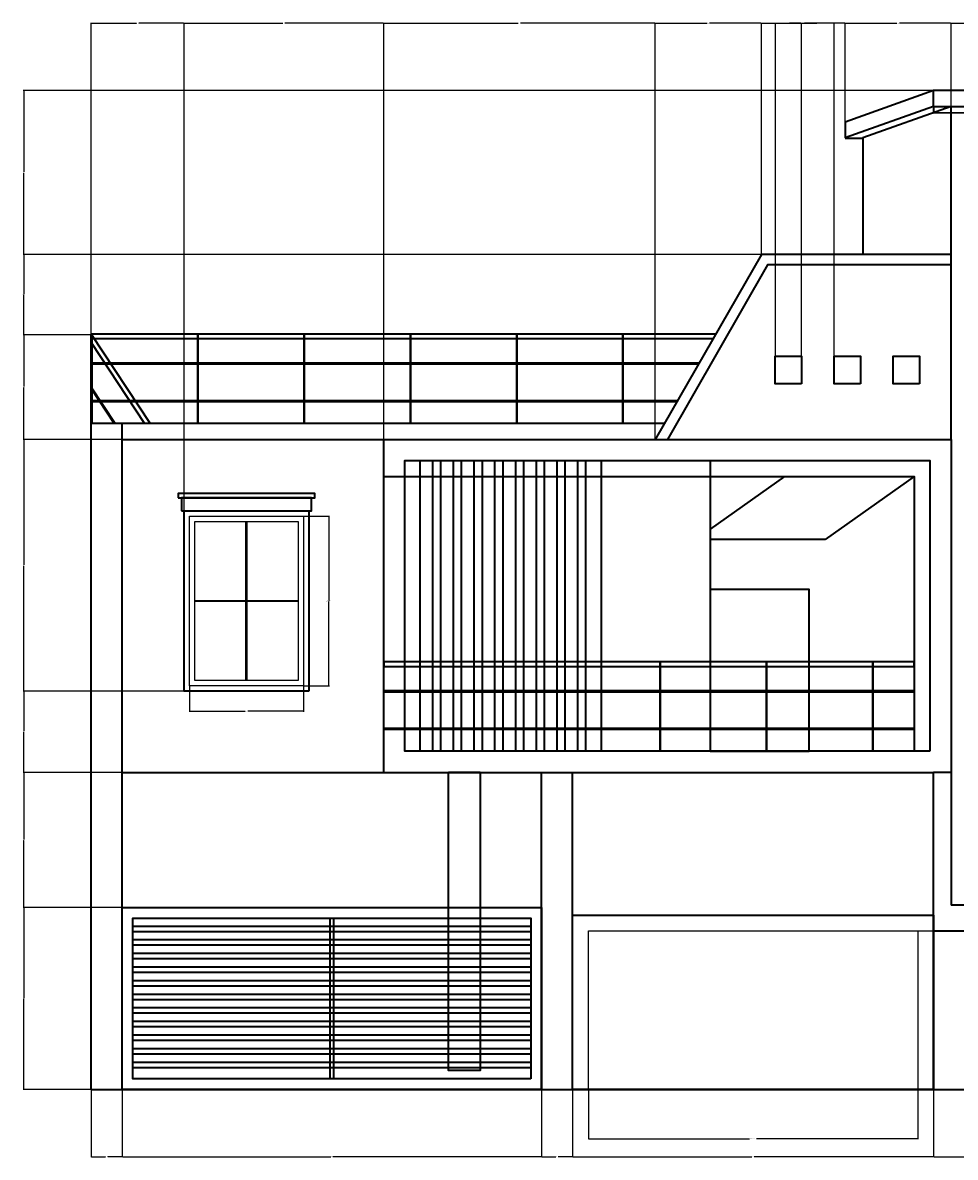
# Model space of a CAD drawing. Units: feet. Extents: x 2415 to 6174, y 866 to 1295.
# Tile 7 of 9: x 3956 to 4309, y 866 to 1295. Entities that reach past the tile are written whole.
import ezdxf

# ---------------------------------------------------------------- set-up
doc = ezdxf.new("R2010")
doc.units = ezdxf.units.FT
for name, color, linetype, lineweight in [('A-ANNO-DIMS', 2, 'Continuous', 18), ('A-DOOR', 4, 'Continuous', 25), ('A-ELEV', 7, 'Continuous', 35), ('A-GLAZ', 4, 'Continuous', 25)]:
    doc.layers.add(name, color=color, linetype=linetype, lineweight=lineweight)
doc.styles.get("Standard").update_dxf_attribs({"font": 'arial.ttf'})
doc.dimstyles.get("Standard").update_dxf_attribs({"dimtxt": 0.18, "dimasz": 0.18, "dimexe": 0.18, "dimexo": 0.0625, "dimgap": 0.09, "dimtad": 0, "dimtih": 1, "dimtoh": 1, "dimdec": 1, "dimzin": 0, "dimdsep": 46, "dimlunit": 3, "dimtxsty": 'Standard', "dimcen": 0.09, "dimadec": 0, "dimazin": 0, "dimtfac": 1, "dimtdec": 1, "dimtofl": 0, "dimtmove": 0, "dimatfit": 3, "dimfxl": 1, "dimtolj": 1, "dimtzin": 0, "dimarcsym": 0})

# ---------------------------------------------------------------- blocks, each defined once
blk = doc.blocks.new('GATE-MAIN')
blk.add_line((0, 60), (124.63, 60))
for points in [[(0, 0), (0, 60)], [(124.63, 60), (124.63, 0)]]:
    blk.add_lwpolyline(points)
blk.add_lwpolyline([(124.63, 0), (0, 0), (0, 60), (124.63, 60)], close=True)
blk = doc.blocks.new('WIN-SMALL')
for points in [[(3333.49, 1044.32), (3290.35, 1044.32), (3290.35, 1108.53), (3333.49, 1108.53)], [(3331.49, 1046.32), (3292.35, 1046.32), (3292.35, 1106.53), (3331.49, 1106.53)], [(3311.72, 1106.53), (3312.12, 1106.53), (3312.12, 1046.32), (3311.72, 1046.32)]]:
    blk.add_lwpolyline(points, close=True)
for points in [[(3292.35, 1076.62), (3331.49, 1076.62)], [(3331.49, 1076.22), (3292.35, 1076.22)]]:
    blk.add_lwpolyline(points)
blk = doc.blocks.new('*D15')
at = {"layer": 'A-ANNO-DIMS', "color": 0, "lineweight": -2, "transparency": 16777216}
for p, q in [((4170.36, 891.54), (4170.36, 872.73)), ((4294.99, 891.54), (4294.99, 872.73)), ((4170.54, 872.91), (4231.36, 872.91)), ((4294.81, 872.91), (4234, 872.91))]:
    blk.add_line(p, q, dxfattribs=at)
at = {"layer": 'A-ANNO-DIMS', "color": 0, "transparency": 16777216}
for points in [[(4170.54, 872.94), (4170.54, 872.88), (4170.36, 872.91)], [(4294.81, 872.94), (4294.81, 872.88), (4294.99, 872.91)]]:
    blk.add_solid(points, dxfattribs=at)
at = {"layer": 'Defpoints', "color": 0, "transparency": 16777216}
for p in [(4170.36, 891.6), (4294.99, 891.6), (4294.99, 872.91)]:
    blk.add_point(p, dxfattribs=at)
at = {"layer": 'A-ANNO-DIMS', "color": 0, "transparency": 16777216, "insert": (4232.68, 872.91), "char_height": 0.18, "attachment_point": 5}
blk.add_mtext('\\A1;MAIN GATE 125 TYP.', dxfattribs=at)
blk = doc.blocks.new('*D16')
at = {"layer": 'A-ANNO-DIMS', "color": 0, "lineweight": -2, "transparency": 16777216}
for p, q in [((4295.05, 951.6), (4313.86, 951.6)), ((4313.68, 951.42), (4313.68, 921.78)), ((4313.68, 891.78), (4313.68, 921.42)), ((4295.05, 891.6), (4313.86, 891.6))]:
    blk.add_line(p, q, dxfattribs=at)
at = {"layer": 'A-ANNO-DIMS', "color": 0, "transparency": 16777216}
for points in [[(4313.65, 951.42), (4313.71, 951.42), (4313.68, 951.6)], [(4313.65, 891.78), (4313.71, 891.78), (4313.68, 891.6)]]:
    blk.add_solid(points, dxfattribs=at)
at = {"layer": 'Defpoints', "color": 0, "transparency": 16777216}
for p in [(4294.99, 951.6), (4313.68, 951.6), (4294.99, 891.6)]:
    blk.add_point(p, dxfattribs=at)
at = {"layer": 'A-ANNO-DIMS', "color": 0, "transparency": 16777216, "insert": (4313.68, 921.6), "char_height": 0.18, "attachment_point": 5}
blk.add_mtext('\\A1;60 TYP.', dxfattribs=at)
blk = doc.blocks.new('*D17')
at = {"layer": 'A-ANNO-DIMS', "color": 0, "lineweight": -2, "transparency": 16777216}
for p, q in [((4062.61, 1108.53), (4072.36, 1108.53)), ((4072.18, 1108.35), (4072.18, 1076.61)), ((4072.18, 1044.5), (4072.18, 1076.24)), ((4062.61, 1044.32), (4072.36, 1044.32))]:
    blk.add_line(p, q, dxfattribs=at)
at = {"layer": 'A-ANNO-DIMS', "color": 0, "transparency": 16777216}
for points in [[(4072.15, 1108.35), (4072.21, 1108.35), (4072.18, 1108.53)], [(4072.15, 1044.5), (4072.21, 1044.5), (4072.18, 1044.32)]]:
    blk.add_solid(points, dxfattribs=at)
at = {"layer": 'Defpoints', "color": 0, "transparency": 16777216}
for p in [(4062.54, 1108.53), (4072.18, 1108.53), (4062.54, 1044.32)]:
    blk.add_point(p, dxfattribs=at)
at = {"layer": 'A-ANNO-DIMS', "color": 0, "transparency": 16777216, "insert": (4072.18, 1076.42), "char_height": 0.18, "attachment_point": 5}
blk.add_mtext('\\A1;WINDOW 64 TYP.', dxfattribs=at)
blk = doc.blocks.new('*D18')
at = {"layer": 'A-ANNO-DIMS', "color": 0, "lineweight": -2, "transparency": 16777216}
for p, q in [((4019.4, 1044.26), (4019.4, 1034.51)), ((4062.54, 1044.26), (4062.54, 1034.51)), ((4019.58, 1034.69), (4040.44, 1034.69)), ((4062.36, 1034.69), (4041.5, 1034.69))]:
    blk.add_line(p, q, dxfattribs=at)
at = {"layer": 'A-ANNO-DIMS', "color": 0, "transparency": 16777216}
for points in [[(4019.58, 1034.72), (4019.58, 1034.66), (4019.4, 1034.69)], [(4062.36, 1034.72), (4062.36, 1034.66), (4062.54, 1034.69)]]:
    blk.add_solid(points, dxfattribs=at)
at = {"layer": 'Defpoints', "color": 0, "transparency": 16777216}
for p in [(4019.4, 1044.32), (4062.54, 1044.32), (4062.54, 1034.69)]:
    blk.add_point(p, dxfattribs=at)
at = {"layer": 'A-ANNO-DIMS', "color": 0, "transparency": 16777216, "insert": (4040.97, 1034.69), "char_height": 0.18, "attachment_point": 5}
blk.add_mtext('\\A1;43 TYP.', dxfattribs=at)
blk = doc.blocks.new('*D19')
at = {"layer": 'A-ANNO-DIMS', "color": 0, "lineweight": -2, "transparency": 16777216}
for p, q in [((3982.18, 891.54), (3982.18, 865.92)), ((3993.97, 891.54), (3993.97, 865.92)), ((3982.36, 866.1), (3987.62, 866.1)), ((3993.79, 866.1), (3988.53, 866.1))]:
    blk.add_line(p, q, dxfattribs=at)
at = {"layer": 'A-ANNO-DIMS', "color": 0, "transparency": 16777216}
for points in [[(3982.36, 866.13), (3982.36, 866.07), (3982.18, 866.1)], [(3993.79, 866.13), (3993.79, 866.07), (3993.97, 866.1)]]:
    blk.add_solid(points, dxfattribs=at)
at = {"layer": 'Defpoints', "color": 0, "transparency": 16777216}
for p in [(3982.18, 891.6), (3993.97, 891.6), (3993.97, 866.1)]:
    blk.add_point(p, dxfattribs=at)
at = {"layer": 'A-ANNO-DIMS', "color": 0, "transparency": 16777216, "insert": (3988.08, 866.1), "char_height": 0.18, "attachment_point": 5}
blk.add_mtext('\\A1;11.787', dxfattribs=at)
blk = doc.blocks.new('*D20')
at = {"layer": 'A-ANNO-DIMS', "color": 0, "lineweight": -2, "transparency": 16777216}
for p, q in [((3993.97, 891.54), (3993.97, 865.92)), ((4152.58, 891.54), (4152.58, 865.92)), ((3994.15, 866.1), (4072.89, 866.1)), ((4152.4, 866.1), (4073.66, 866.1))]:
    blk.add_line(p, q, dxfattribs=at)
at = {"layer": 'A-ANNO-DIMS', "color": 0, "transparency": 16777216}
for points in [[(3994.15, 866.13), (3994.15, 866.07), (3993.97, 866.1)], [(4152.4, 866.13), (4152.4, 866.07), (4152.58, 866.1)]]:
    blk.add_solid(points, dxfattribs=at)
at = {"layer": 'Defpoints', "color": 0, "transparency": 16777216}
for p in [(3993.97, 891.6), (4152.58, 891.6), (4152.58, 866.1)]:
    blk.add_point(p, dxfattribs=at)
at = {"layer": 'A-ANNO-DIMS', "color": 0, "transparency": 16777216, "insert": (4073.27, 866.1), "char_height": 0.18, "attachment_point": 5}
blk.add_mtext('\\A1;158.6', dxfattribs=at)
blk = doc.blocks.new('*D21')
at = {"layer": 'A-ANNO-DIMS', "color": 0, "lineweight": -2, "transparency": 16777216}
for p, q in [((4152.58, 891.54), (4152.58, 865.92)), ((4164.36, 891.54), (4164.36, 865.92)), ((4152.76, 866.1), (4158.01, 866.1)), ((4164.18, 866.1), (4158.93, 866.1))]:
    blk.add_line(p, q, dxfattribs=at)
at = {"layer": 'A-ANNO-DIMS', "color": 0, "transparency": 16777216}
for points in [[(4152.76, 866.13), (4152.76, 866.07), (4152.58, 866.1)], [(4164.18, 866.13), (4164.18, 866.07), (4164.36, 866.1)]]:
    blk.add_solid(points, dxfattribs=at)
at = {"layer": 'Defpoints', "color": 0, "transparency": 16777216}
for p in [(4152.58, 891.6), (4164.36, 891.6), (4164.36, 866.1)]:
    blk.add_point(p, dxfattribs=at)
at = {"layer": 'A-ANNO-DIMS', "color": 0, "transparency": 16777216, "insert": (4158.47, 866.1), "char_height": 0.18, "attachment_point": 5}
blk.add_mtext('\\A1;11.787', dxfattribs=at)
blk = doc.blocks.new('*D22')
at = {"layer": 'A-ANNO-DIMS', "color": 0, "lineweight": -2, "transparency": 16777216}
for p, q in [((4164.36, 891.54), (4164.36, 865.92)), ((4300.99, 891.54), (4300.99, 865.92)), ((4164.54, 866.1), (4232.22, 866.1)), ((4300.81, 866.1), (4233.13, 866.1))]:
    blk.add_line(p, q, dxfattribs=at)
at = {"layer": 'A-ANNO-DIMS', "color": 0, "transparency": 16777216}
for points in [[(4164.54, 866.13), (4164.54, 866.07), (4164.36, 866.1)], [(4300.81, 866.13), (4300.81, 866.07), (4300.99, 866.1)]]:
    blk.add_solid(points, dxfattribs=at)
at = {"layer": 'Defpoints', "color": 0, "transparency": 16777216}
for p in [(4164.36, 891.6), (4300.99, 891.6), (4300.99, 866.1)]:
    blk.add_point(p, dxfattribs=at)
at = {"layer": 'A-ANNO-DIMS', "color": 0, "transparency": 16777216, "insert": (4232.68, 866.1), "char_height": 0.18, "attachment_point": 5}
blk.add_mtext('\\A1;136.63', dxfattribs=at)
blk = doc.blocks.new('*D23')
at = {"layer": 'A-ANNO-DIMS', "color": 0, "lineweight": -2, "transparency": 16777216}
for p, q in [((4300.99, 891.54), (4300.99, 865.92)), ((4330.05, 891.54), (4330.05, 865.92)), ((4301.17, 866.1), (4315.13, 866.1)), ((4329.87, 866.1), (4315.92, 866.1))]:
    blk.add_line(p, q, dxfattribs=at)
at = {"layer": 'A-ANNO-DIMS', "color": 0, "transparency": 16777216}
for points in [[(4301.17, 866.13), (4301.17, 866.07), (4300.99, 866.1)], [(4329.87, 866.13), (4329.87, 866.07), (4330.05, 866.1)]]:
    blk.add_solid(points, dxfattribs=at)
at = {"layer": 'Defpoints', "color": 0, "transparency": 16777216}
for p in [(4300.99, 891.6), (4330.05, 891.6), (4330.05, 866.1)]:
    blk.add_point(p, dxfattribs=at)
at = {"layer": 'A-ANNO-DIMS', "color": 0, "transparency": 16777216, "insert": (4315.52, 866.1), "char_height": 0.18, "attachment_point": 5}
blk.add_mtext('\\A1;29.06', dxfattribs=at)
blk = doc.blocks.new('*D27')
at = {"layer": 'A-ANNO-DIMS', "color": 0, "lineweight": -2, "transparency": 16777216}
for p, q in [((3982.18, 1177.2), (3982.18, 1295.28)), ((3982.36, 1295.1), (3999.33, 1295.1)), ((4017.22, 1295.1), (4000.26, 1295.1)), ((4017.4, 1042.38), (4017.4, 1295.28))]:
    blk.add_line(p, q, dxfattribs=at)
at = {"layer": 'A-ANNO-DIMS', "color": 0, "transparency": 16777216}
for points in [[(3982.36, 1295.13), (3982.36, 1295.07), (3982.18, 1295.1)], [(4017.22, 1295.13), (4017.22, 1295.07), (4017.4, 1295.1)]]:
    blk.add_solid(points, dxfattribs=at)
at = {"layer": 'Defpoints', "color": 0, "transparency": 16777216}
for p in [(4017.4, 1295.1), (3982.18, 1177.14), (4017.4, 1042.32)]:
    blk.add_point(p, dxfattribs=at)
at = {"layer": 'A-ANNO-DIMS', "color": 0, "transparency": 16777216, "insert": (3999.79, 1295.1), "char_height": 0.18, "attachment_point": 5}
blk.add_mtext('\\A1;35.216', dxfattribs=at)
blk = doc.blocks.new('*D28')
at = {"layer": 'A-ANNO-DIMS', "color": 0, "lineweight": -2, "transparency": 16777216}
for p, q in [((4017.4, 1042.38), (4017.4, 1295.28)), ((4017.58, 1295.1), (4054.77, 1295.1)), ((4092.74, 1295.1), (4055.55, 1295.1)), ((4092.92, 1137.66), (4092.92, 1295.28))]:
    blk.add_line(p, q, dxfattribs=at)
at = {"layer": 'A-ANNO-DIMS', "color": 0, "transparency": 16777216}
for points in [[(4017.58, 1295.13), (4017.58, 1295.07), (4017.4, 1295.1)], [(4092.74, 1295.13), (4092.74, 1295.07), (4092.92, 1295.1)]]:
    blk.add_solid(points, dxfattribs=at)
at = {"layer": 'Defpoints', "color": 0, "transparency": 16777216}
for p in [(4092.92, 1295.1), (4092.92, 1137.6), (4017.4, 1042.32)]:
    blk.add_point(p, dxfattribs=at)
at = {"layer": 'A-ANNO-DIMS', "color": 0, "transparency": 16777216, "insert": (4055.16, 1295.1), "char_height": 0.18, "attachment_point": 5}
blk.add_mtext('\\A1;75.52', dxfattribs=at)
blk = doc.blocks.new('*D29')
at = {"layer": 'A-ANNO-DIMS', "color": 0, "lineweight": -2, "transparency": 16777216}
for p, q in [((4092.92, 1137.66), (4092.92, 1295.28)), ((4093.1, 1295.1), (4143.83, 1295.1)), ((4195.48, 1295.1), (4144.74, 1295.1)), ((4195.66, 1137.66), (4195.66, 1295.28))]:
    blk.add_line(p, q, dxfattribs=at)
at = {"layer": 'A-ANNO-DIMS', "color": 0, "transparency": 16777216}
for points in [[(4093.1, 1295.13), (4093.1, 1295.07), (4092.92, 1295.1)], [(4195.48, 1295.13), (4195.48, 1295.07), (4195.66, 1295.1)]]:
    blk.add_solid(points, dxfattribs=at)
at = {"layer": 'Defpoints', "color": 0, "transparency": 16777216}
for p in [(4195.66, 1295.1), (4092.92, 1137.6), (4195.66, 1137.6)]:
    blk.add_point(p, dxfattribs=at)
at = {"layer": 'A-ANNO-DIMS', "color": 0, "transparency": 16777216, "insert": (4144.29, 1295.1), "char_height": 0.18, "attachment_point": 5}
blk.add_mtext('\\A1;102.73', dxfattribs=at)
blk = doc.blocks.new('*D30')
at = {"layer": 'A-ANNO-DIMS', "color": 0, "lineweight": -2, "transparency": 16777216}
for p, q in [((4195.66, 1137.66), (4195.66, 1295.28)), ((4195.84, 1295.1), (4215.35, 1295.1)), ((4235.67, 1295.1), (4216.15, 1295.1)), ((4235.85, 1207.66), (4235.85, 1295.28))]:
    blk.add_line(p, q, dxfattribs=at)
at = {"layer": 'A-ANNO-DIMS', "color": 0, "transparency": 16777216}
for points in [[(4195.84, 1295.13), (4195.84, 1295.07), (4195.66, 1295.1)], [(4235.67, 1295.13), (4235.67, 1295.07), (4235.85, 1295.1)]]:
    blk.add_solid(points, dxfattribs=at)
at = {"layer": 'Defpoints', "color": 0, "transparency": 16777216}
for p in [(4235.85, 1295.1), (4235.85, 1207.6), (4195.66, 1137.6)]:
    blk.add_point(p, dxfattribs=at)
at = {"layer": 'A-ANNO-DIMS', "color": 0, "transparency": 16777216, "insert": (4215.75, 1295.1), "char_height": 0.18, "attachment_point": 5}
blk.add_mtext('\\A1;40.19', dxfattribs=at)
blk = doc.blocks.new('*D31')
at = {"layer": 'A-ANNO-DIMS', "color": 0, "lineweight": -2, "transparency": 16777216}
for p, q in [((4235.85, 1207.66), (4235.85, 1295.28)), ((4236.03, 1295.1), (4251.31, 1295.1)), ((4267.39, 1295.1), (4252.1, 1295.1)), ((4267.57, 1257.71), (4267.57, 1295.28))]:
    blk.add_line(p, q, dxfattribs=at)
at = {"layer": 'A-ANNO-DIMS', "color": 0, "transparency": 16777216}
for points in [[(4236.03, 1295.13), (4236.03, 1295.07), (4235.85, 1295.1)], [(4267.39, 1295.13), (4267.39, 1295.07), (4267.57, 1295.1)]]:
    blk.add_solid(points, dxfattribs=at)
at = {"layer": 'Defpoints', "color": 0, "transparency": 16777216}
for p in [(4267.57, 1295.1), (4267.57, 1257.64), (4235.85, 1207.6)]:
    blk.add_point(p, dxfattribs=at)
at = {"layer": 'A-ANNO-DIMS', "color": 0, "transparency": 16777216, "insert": (4251.71, 1295.1), "char_height": 0.18, "attachment_point": 5}
blk.add_mtext('\\A1;31.72', dxfattribs=at)
blk = doc.blocks.new('*D32')
at = {"layer": 'A-ANNO-DIMS', "color": 0, "lineweight": -2, "transparency": 16777216}
for p, q in [((4267.57, 1257.71), (4267.57, 1295.28)), ((4267.75, 1295.1), (4287.12, 1295.1)), ((4307.43, 1295.1), (4288.06, 1295.1)), ((4307.61, 1263.66), (4307.61, 1295.28))]:
    blk.add_line(p, q, dxfattribs=at)
at = {"layer": 'A-ANNO-DIMS', "color": 0, "transparency": 16777216}
for points in [[(4267.75, 1295.13), (4267.75, 1295.07), (4267.57, 1295.1)], [(4307.43, 1295.13), (4307.43, 1295.07), (4307.61, 1295.1)]]:
    blk.add_solid(points, dxfattribs=at)
at = {"layer": 'Defpoints', "color": 0, "transparency": 16777216}
for p in [(4307.61, 1295.1), (4307.61, 1263.6), (4267.57, 1257.64)]:
    blk.add_point(p, dxfattribs=at)
at = {"layer": 'A-ANNO-DIMS', "color": 0, "transparency": 16777216, "insert": (4287.59, 1295.1), "char_height": 0.18, "attachment_point": 5}
blk.add_mtext('\\A1;40.046', dxfattribs=at)
blk = doc.blocks.new('*D33')
at = {"layer": 'A-ANNO-DIMS', "color": 0, "lineweight": -2, "transparency": 16777216}
for p, q in [((4307.61, 1263.66), (4307.61, 1295.28)), ((4307.79, 1295.1), (4318.98, 1295.1)), ((4331.09, 1295.1), (4319.91, 1295.1)), ((4331.27, 1239.13), (4331.27, 1295.28))]:
    blk.add_line(p, q, dxfattribs=at)
at = {"layer": 'A-ANNO-DIMS', "color": 0, "transparency": 16777216}
for points in [[(4307.79, 1295.13), (4307.79, 1295.07), (4307.61, 1295.1)], [(4331.09, 1295.13), (4331.09, 1295.07), (4331.27, 1295.1)]]:
    blk.add_solid(points, dxfattribs=at)
at = {"layer": 'Defpoints', "color": 0, "transparency": 16777216}
for p in [(4331.27, 1295.1), (4307.61, 1263.6), (4331.27, 1239.07)]:
    blk.add_point(p, dxfattribs=at)
at = {"layer": 'A-ANNO-DIMS', "color": 0, "transparency": 16777216, "insert": (4319.44, 1295.1), "char_height": 0.18, "attachment_point": 5}
blk.add_mtext('\\A1;23.657', dxfattribs=at)
blk = doc.blocks.new('*D38')
at = {"layer": 'A-ANNO-DIMS', "color": 0, "lineweight": -2, "transparency": 16777216}
for p, q in [((3993.91, 960.43), (3956.5, 960.43)), ((3956.68, 960.25), (3956.68, 926.2)), ((3956.68, 891.78), (3956.68, 925.83)), ((3993.91, 891.6), (3956.5, 891.6))]:
    blk.add_line(p, q, dxfattribs=at)
at = {"layer": 'A-ANNO-DIMS', "color": 0, "transparency": 16777216}
for points in [[(3956.65, 960.25), (3956.71, 960.25), (3956.68, 960.43)], [(3956.65, 891.78), (3956.71, 891.78), (3956.68, 891.6)]]:
    blk.add_solid(points, dxfattribs=at)
at = {"layer": 'Defpoints', "color": 0, "transparency": 16777216}
for p in [(3956.68, 960.43), (3993.97, 960.43), (3993.97, 891.6)]:
    blk.add_point(p, dxfattribs=at)
at = {"layer": 'A-ANNO-DIMS', "color": 0, "transparency": 16777216, "insert": (3956.68, 926.02), "char_height": 0.18, "attachment_point": 5}
blk.add_mtext('\\A1;68.83', dxfattribs=at)
blk = doc.blocks.new('*D39')
at = {"layer": 'A-ANNO-DIMS', "color": 0, "lineweight": -2, "transparency": 16777216}
for p, q in [((3993.91, 1011.6), (3956.5, 1011.6)), ((3956.68, 1011.42), (3956.68, 986.2)), ((3956.68, 960.61), (3956.68, 985.83)), ((3993.91, 960.43), (3956.5, 960.43))]:
    blk.add_line(p, q, dxfattribs=at)
at = {"layer": 'A-ANNO-DIMS', "color": 0, "transparency": 16777216}
for points in [[(3956.65, 1011.42), (3956.71, 1011.42), (3956.68, 1011.6)], [(3956.65, 960.61), (3956.71, 960.61), (3956.68, 960.43)]]:
    blk.add_solid(points, dxfattribs=at)
at = {"layer": 'Defpoints', "color": 0, "transparency": 16777216}
for p in [(3956.68, 1011.6), (3993.97, 1011.6), (3993.97, 960.43)]:
    blk.add_point(p, dxfattribs=at)
at = {"layer": 'A-ANNO-DIMS', "color": 0, "transparency": 16777216, "insert": (3956.68, 986.02), "char_height": 0.18, "attachment_point": 5}
blk.add_mtext('\\A1;51.17', dxfattribs=at)
blk = doc.blocks.new('*D40')
at = {"layer": 'A-ANNO-DIMS', "color": 0, "lineweight": -2, "transparency": 16777216}
for p, q in [((4017.34, 1042.32), (3956.5, 1042.32)), ((3956.68, 1042.14), (3956.68, 1027.14)), ((3956.68, 1011.78), (3956.68, 1026.78)), ((3993.91, 1011.6), (3956.5, 1011.6))]:
    blk.add_line(p, q, dxfattribs=at)
at = {"layer": 'A-ANNO-DIMS', "color": 0, "transparency": 16777216}
for points in [[(3956.65, 1042.14), (3956.71, 1042.14), (3956.68, 1042.32)], [(3956.65, 1011.78), (3956.71, 1011.78), (3956.68, 1011.6)]]:
    blk.add_solid(points, dxfattribs=at)
at = {"layer": 'Defpoints', "color": 0, "transparency": 16777216}
for p in [(3956.68, 1042.32), (4017.4, 1042.32), (3993.97, 1011.6)]:
    blk.add_point(p, dxfattribs=at)
at = {"layer": 'A-ANNO-DIMS', "color": 0, "transparency": 16777216, "insert": (3956.68, 1026.96), "char_height": 0.18, "attachment_point": 5}
blk.add_mtext('\\A1;30.72', dxfattribs=at)
blk = doc.blocks.new('*D41')
at = {"layer": 'A-ANNO-DIMS', "color": 0, "lineweight": -2, "transparency": 16777216}
for p, q in [((4092.86, 1137.6), (3956.5, 1137.6)), ((3956.68, 1137.42), (3956.68, 1090.14)), ((3956.68, 1042.5), (3956.68, 1089.78)), ((4017.34, 1042.32), (3956.5, 1042.32))]:
    blk.add_line(p, q, dxfattribs=at)
at = {"layer": 'A-ANNO-DIMS', "color": 0, "transparency": 16777216}
for points in [[(3956.65, 1137.42), (3956.71, 1137.42), (3956.68, 1137.6)], [(3956.65, 1042.5), (3956.71, 1042.5), (3956.68, 1042.32)]]:
    blk.add_solid(points, dxfattribs=at)
at = {"layer": 'Defpoints', "color": 0, "transparency": 16777216}
for p in [(3956.68, 1137.6), (4092.92, 1137.6), (4017.4, 1042.32)]:
    blk.add_point(p, dxfattribs=at)
at = {"layer": 'A-ANNO-DIMS', "color": 0, "transparency": 16777216, "insert": (3956.68, 1089.96), "char_height": 0.18, "attachment_point": 5}
blk.add_mtext('\\A1;95.28', dxfattribs=at)
blk = doc.blocks.new('*D42')
at = {"layer": 'A-ANNO-DIMS', "color": 0, "lineweight": -2, "transparency": 16777216}
for p, q in [((3982.12, 1177.14), (3956.5, 1177.14)), ((3956.68, 1176.96), (3956.68, 1157.55)), ((3956.68, 1137.78), (3956.68, 1157.19)), ((4092.86, 1137.6), (3956.5, 1137.6))]:
    blk.add_line(p, q, dxfattribs=at)
at = {"layer": 'A-ANNO-DIMS', "color": 0, "transparency": 16777216}
for points in [[(3956.65, 1176.96), (3956.71, 1176.96), (3956.68, 1177.14)], [(3956.65, 1137.78), (3956.71, 1137.78), (3956.68, 1137.6)]]:
    blk.add_solid(points, dxfattribs=at)
at = {"layer": 'Defpoints', "color": 0, "transparency": 16777216}
for p in [(3956.68, 1177.14), (3982.18, 1177.14), (4092.92, 1137.6)]:
    blk.add_point(p, dxfattribs=at)
at = {"layer": 'A-ANNO-DIMS', "color": 0, "transparency": 16777216, "insert": (3956.68, 1157.37), "char_height": 0.18, "attachment_point": 5}
blk.add_mtext('\\A1;39.54', dxfattribs=at)
blk = doc.blocks.new('*D43')
at = {"layer": 'A-ANNO-DIMS', "color": 0, "lineweight": -2, "transparency": 16777216}
for p, q in [((4235.78, 1207.6), (3956.5, 1207.6)), ((3956.68, 1207.42), (3956.68, 1192.55)), ((3956.68, 1177.32), (3956.68, 1192.19)), ((3982.12, 1177.14), (3956.5, 1177.14))]:
    blk.add_line(p, q, dxfattribs=at)
at = {"layer": 'A-ANNO-DIMS', "color": 0, "transparency": 16777216}
for points in [[(3956.65, 1207.42), (3956.71, 1207.42), (3956.68, 1207.6)], [(3956.65, 1177.32), (3956.71, 1177.32), (3956.68, 1177.14)]]:
    blk.add_solid(points, dxfattribs=at)
at = {"layer": 'Defpoints', "color": 0, "transparency": 16777216}
for p in [(3956.68, 1207.6), (4235.85, 1207.6), (3982.18, 1177.14)]:
    blk.add_point(p, dxfattribs=at)
at = {"layer": 'A-ANNO-DIMS', "color": 0, "transparency": 16777216, "insert": (3956.68, 1192.37), "char_height": 0.18, "attachment_point": 5}
blk.add_mtext('\\A1;30.457', dxfattribs=at)
blk = doc.blocks.new('*D44')
at = {"layer": 'A-ANNO-DIMS', "color": 0, "lineweight": -2, "transparency": 16777216}
for p, q in [((4300.93, 1269.6), (3956.5, 1269.6)), ((3956.68, 1269.42), (3956.68, 1238.78)), ((3956.68, 1207.78), (3956.68, 1238.42)), ((4235.78, 1207.6), (3956.5, 1207.6))]:
    blk.add_line(p, q, dxfattribs=at)
at = {"layer": 'A-ANNO-DIMS', "color": 0, "transparency": 16777216}
for points in [[(3956.65, 1269.42), (3956.71, 1269.42), (3956.68, 1269.6)], [(3956.65, 1207.78), (3956.71, 1207.78), (3956.68, 1207.6)]]:
    blk.add_solid(points, dxfattribs=at)
at = {"layer": 'Defpoints', "color": 0, "transparency": 16777216}
for p in [(3956.68, 1269.6), (4300.99, 1269.6), (4235.85, 1207.6)]:
    blk.add_point(p, dxfattribs=at)
at = {"layer": 'A-ANNO-DIMS', "color": 0, "transparency": 16777216, "insert": (3956.68, 1238.6), "char_height": 0.18, "attachment_point": 5}
blk.add_mtext('\\A1;62', dxfattribs=at)
blk = doc.blocks.new('*D51')
at = {"layer": 'A-ANNO-DIMS', "color": 0, "lineweight": -2, "transparency": 16777216}
for p, q in [((4241.11, 1169.09), (4241.11, 1295.28)), ((4241.29, 1295.1), (4245.66, 1295.1)), ((4250.81, 1295.1), (4246.44, 1295.1)), ((4250.99, 1169.09), (4250.99, 1295.28))]:
    blk.add_line(p, q, dxfattribs=at)
at = {"layer": 'A-ANNO-DIMS', "color": 0, "transparency": 16777216}
for points in [[(4241.29, 1295.13), (4241.29, 1295.07), (4241.11, 1295.1)], [(4250.81, 1295.13), (4250.81, 1295.07), (4250.99, 1295.1)]]:
    blk.add_solid(points, dxfattribs=at)
at = {"layer": 'Defpoints', "color": 0, "transparency": 16777216}
for p in [(4250.99, 1295.1), (4241.11, 1169.03), (4250.99, 1169.03)]:
    blk.add_point(p, dxfattribs=at)
at = {"layer": 'A-ANNO-DIMS', "color": 0, "transparency": 16777216, "insert": (4246.05, 1295.1), "char_height": 0.18, "attachment_point": 5}
blk.add_mtext('\\A1;9.886', dxfattribs=at)
blk = doc.blocks.new('*D52')
at = {"layer": 'A-ANNO-DIMS', "color": 0, "lineweight": -2, "transparency": 16777216}
for p, q in [((4250.99, 1158.74), (4250.99, 1295.28)), ((4251.17, 1295.1), (4256.76, 1295.1)), ((4263.25, 1295.1), (4257.67, 1295.1)), ((4263.43, 1158.74), (4263.43, 1295.28))]:
    blk.add_line(p, q, dxfattribs=at)
at = {"layer": 'A-ANNO-DIMS', "color": 0, "transparency": 16777216}
for points in [[(4251.17, 1295.13), (4251.17, 1295.07), (4250.99, 1295.1)], [(4263.25, 1295.13), (4263.25, 1295.07), (4263.43, 1295.1)]]:
    blk.add_solid(points, dxfattribs=at)
at = {"layer": 'Defpoints', "color": 0, "transparency": 16777216}
for p in [(4263.43, 1295.1), (4250.99, 1158.67), (4263.43, 1158.67)]:
    blk.add_point(p, dxfattribs=at)
at = {"layer": 'A-ANNO-DIMS', "color": 0, "transparency": 16777216, "insert": (4257.21, 1295.1), "char_height": 0.18, "attachment_point": 5}
blk.add_mtext('\\A1;12.438', dxfattribs=at)

msp = doc.modelspace()

# ---------------------------------------------------------------- linework, layer by layer
at = {"layer": 'A-ELEV'}
for p, q in [((4300.9903, 1269.5992), (4267.5678, 1257.6449)), ((4419.1468, 1269.5992), (4300.9903, 1269.5992)), ((4300.9903, 1263.5992), (4300.9903, 1269.5992)), ((4300.9903, 1263.5992), (4267.5678, 1251.6449)), ((4307.6134, 1263.5992), (4274.1909, 1251.6449)), ((4300.9903, 1263.5992), (4419.1468, 1263.5992)), ((4300.9903, 1263.5992), (4300.9903, 1261.2303)), ((4307.6134, 1137.5992), (4307.6134, 1263.5992)), ((4300.9903, 1261.2303), (4411.1278, 1261.2628)), ((4267.5678, 1257.6449), (4267.5678, 1251.6449)), ((4267.5678, 1251.6449), (4267.6022, 1251.5295)), ((4267.5678, 1251.5295), (4274.1909, 1251.5295)), ((4273.8049, 1251.5295), (4274.1909, 1251.6449)), ((4274.1909, 1251.6449), (4274.1909, 1207.5992)), ((3982.1845, 1143.5993), (3982.1845, 1177.4585)), ((3982.1845, 1177.4585), (4004.5183, 1143.5993)), ((3982.1845, 891.5992), (3982.1845, 1143.5993)), ((3993.9716, 1143.5993), (3982.1845, 1143.5993)), ((4199.1004, 1143.5993), (3993.9716, 1143.5993)), ((3993.9716, 1137.5992), (4307.6134, 1137.5992)), ((4092.9223, 1011.5992), (4092.9223, 1137.5992)), ((4307.6134, 1137.5992), (4307.6134, 961.3655)), ((4216.4986, 1129.5993), (4216.4986, 1019.5993)), ((4244.6046, 1123.5993), (4216.4986, 1103.5745)), ((4293.6134, 1123.5993), (4260.0013, 1099.6515)), ((4260.0013, 1099.6515), (4216.4986, 1099.6515)), ((3993.9716, 1011.5992), (4300.9903, 1011.5992)), ((4152.5764, 891.5992), (4152.5764, 1011.5992)), ((4164.3635, 891.5992), (4164.3635, 1011.5992)), ((4300.9903, 891.5992), (4300.9903, 1011.5992)), ((4164.3635, 957.5993), (4300.9903, 957.5993)), ((4300.9903, 951.5993), (4330.0513, 951.5993)), ((3982.1845, 891.5992), (4462.1845, 891.5992))]:
    msp.add_line(p, q, dxfattribs=at)
for points in [[(4411.1278, 1263.5992), (4411.1278, 961.3655), (4307.6134, 961.3655)], [(4307.6134, 1207.5992), (4235.8465, 1207.5992), (4195.6555, 1137.5992)], [(4307.6134, 1203.5993), (4238.1623, 1203.5993), (4200.2679, 1137.5992)], [(4218.541, 1177.4585), (3982.1845, 1177.4585)], [(3982.1845, 1177.1423), (3982.3299, 1177.2382)], [(3982.3071, 1177.4585), (3982.3071, 1143.5993)], [(3982.5711, 1143.5993), (3982.5711, 1177.4585)], [(4022.507, 1177.4585), (4022.507, 1143.5993)], [(4022.7709, 1143.5993), (4022.7709, 1177.4585)], [(4062.7068, 1177.4585), (4062.7068, 1143.5993)], [(4062.9707, 1143.5993), (4062.9707, 1177.4585)], [(4102.9066, 1177.4585), (4102.9066, 1143.5993)], [(4103.1705, 1143.5993), (4103.1705, 1177.4585)], [(4143.1065, 1177.4585), (4143.1065, 1143.5993)], [(4143.3704, 1143.5993), (4143.3704, 1177.4585)], [(4183.3063, 1177.4585), (4183.3063, 1143.5993)], [(4183.5702, 1143.5993), (4183.5702, 1177.4585)], [(3982.1845, 1175.7117), (4217.5381, 1175.7117)], [(3982.1845, 1174.2861), (4002.4258, 1143.5993)], [(4212.1844, 1166.3873), (3982.1845, 1166.3873)], [(3982.1845, 1166.1234), (4212.0328, 1166.1234)], [(3991.2557, 1143.5993), (3982.1845, 1157.3516)], [(3982.1845, 1156.8722), (3990.9395, 1143.5993)], [(4204.054, 1152.2269), (3982.1845, 1152.2269)], [(3982.1845, 1151.963), (4203.9025, 1151.963)], [(3982.1845, 891.5992), (3993.9716, 891.5992), (3993.9716, 1143.5993)], [(4004.3191, 1143.9012), (4003.8613, 1143.5993)], [(4004.3406, 1143.5993), (4004.4644, 1143.6809)], [(4307.6134, 1137.5992), (4307.6134, 1137.5992), (4307.6134, 1011.5992), (4300.9903, 1011.5992)], [(4092.9223, 1123.5993), (4293.6134, 1123.5993), (4293.6134, 1019.5993)], [(4197.4197, 1053.4585), (4197.4197, 1019.5993)], [(4197.6836, 1019.5993), (4197.6836, 1053.4585)], [(4237.6195, 1053.4585), (4237.6195, 1019.5993)], [(4237.8834, 1019.5993), (4237.8834, 1053.4585)], [(4277.8193, 1053.4585), (4277.8193, 1019.5993)], [(4278.0833, 1019.5993), (4278.0833, 1053.4585)], [(4129.3889, 1011.5992), (4117.4977, 1011.5992)], [(4129.3889, 1011.5992), (4129.3889, 898.815), (4117.4977, 898.815), (4117.4977, 1011.5992)], [(4152.5764, 891.5992), (4164.3635, 891.5992)], [(4300.9903, 891.5992), (4164.3635, 891.5992)]]:
    msp.add_lwpolyline(points, dxfattribs=at)
for points in [[(4250.9935, 1158.6726), (4241.1072, 1158.6726), (4241.1072, 1169.0289), (4250.9935, 1169.0289)], [(4273.3172, 1158.6726), (4263.431, 1158.6726), (4263.431, 1169.0289), (4273.3172, 1169.0289)], [(4295.6409, 1158.6726), (4285.7547, 1158.6726), (4285.7547, 1169.0289), (4295.6409, 1169.0289)], [(4299.6134, 1019.5993), (4100.9223, 1019.5993), (4100.9223, 1129.5993), (4299.6134, 1129.5993)], [(4106.7136, 1129.5993), (4111.366, 1129.5993), (4111.366, 1019.5993), (4106.7136, 1019.5993)], [(4114.5562, 1129.5993), (4119.2086, 1129.5993), (4119.2086, 1019.5993), (4114.5562, 1019.5993)], [(4122.3988, 1129.5993), (4127.0512, 1129.5993), (4127.0512, 1019.5993), (4122.3988, 1019.5993)], [(4130.2414, 1129.5993), (4134.8938, 1129.5993), (4134.8938, 1019.5993), (4130.2414, 1019.5993)], [(4138.084, 1129.5993), (4142.7364, 1129.5993), (4142.7364, 1019.5993), (4138.084, 1019.5993)], [(4145.9266, 1129.5993), (4150.579, 1129.5993), (4150.579, 1019.5993), (4145.9266, 1019.5993)], [(4153.7692, 1129.5993), (4158.4216, 1129.5993), (4158.4216, 1019.5993), (4153.7692, 1019.5993)], [(4161.6118, 1129.5993), (4166.2642, 1129.5993), (4166.2642, 1019.5993), (4161.6118, 1019.5993)], [(4169.3758, 1129.5993), (4175.209, 1129.5993), (4175.209, 1019.5993), (4169.3758, 1019.5993)], [(4015.0985, 1115.4381), (4066.846, 1115.4381), (4066.846, 1117.0591), (4015.0985, 1117.0591)], [(4016.3575, 1110.528), (4065.587, 1110.528), (4065.587, 1115.4381), (4016.3575, 1115.4381)], [(4064.5437, 1042.3194), (4017.4008, 1042.3194), (4017.4008, 1110.528), (4064.5437, 1110.528)], [(4216.4986, 1019.5993), (4253.8568, 1019.5993), (4253.8568, 1080.8275), (4216.4986, 1080.8275)], [(4293.6134, 1053.4585), (4092.9223, 1053.4585), (4092.9223, 1051.7117), (4293.6134, 1051.7117)], [(4293.6134, 1042.3873), (4092.9223, 1042.3873), (4092.9223, 1042.1234), (4293.6134, 1042.1234)], [(4293.6134, 1028.2269), (4092.9223, 1028.2269), (4092.9223, 1027.963), (4293.6134, 1027.963)], [(4152.5764, 891.5992), (3993.9716, 891.5992), (3993.9716, 960.433), (4152.5764, 960.433)], [(4300.9903, 891.5992), (4164.3635, 891.5992), (4164.3635, 957.5993), (4300.9903, 957.5993)], [(4148.5764, 895.5993), (3997.9716, 895.5993), (3997.9716, 956.433), (4148.5764, 956.433)], [(3997.9716, 953.4503), (4148.5764, 953.4503), (4148.5764, 951.2861), (3997.9716, 951.2861)], [(4072.6433, 956.433), (4073.9048, 956.433), (4073.9048, 895.5993), (4072.6433, 895.5993)], [(3997.9716, 948.3033), (4148.5764, 948.3033), (4148.5764, 946.1391), (3997.9716, 946.1391)], [(3997.9716, 943.1563), (4148.5764, 943.1563), (4148.5764, 940.9922), (3997.9716, 940.9922)], [(3997.9716, 938.0094), (4148.5764, 938.0094), (4148.5764, 935.8452), (3997.9716, 935.8452)], [(3997.9716, 932.8624), (4148.5764, 932.8624), (4148.5764, 930.6983), (3997.9716, 930.6983)], [(3997.9716, 927.7155), (4148.5764, 927.7155), (4148.5764, 925.5513), (3997.9716, 925.5513)], [(3997.9716, 922.5685), (4148.5764, 922.5685), (4148.5764, 920.4043), (3997.9716, 920.4043)], [(3997.9716, 917.4215), (4148.5764, 917.4215), (4148.5764, 915.2574), (3997.9716, 915.2574)], [(3997.9716, 912.2746), (4148.5764, 912.2746), (4148.5764, 910.1104), (3997.9716, 910.1104)], [(3997.9716, 907.1276), (4148.5764, 907.1276), (4148.5764, 904.9635), (3997.9716, 904.9635)], [(3997.9716, 901.9807), (4148.5764, 901.9807), (4148.5764, 899.8165), (3997.9716, 899.8165)]]:
    msp.add_lwpolyline(points, close=True, dxfattribs=at)

# ---------------------------------------------------------------- block references
at = {"layer": 'A-DOOR'}
msp.add_blockref('GATE-MAIN', (4170.3636, 891.599), dxfattribs=at)
at = {"layer": 'A-GLAZ'}
msp.add_blockref('WIN-SMALL', (729.0556, 0), dxfattribs=at)

# ---------------------------------------------------------------- dimensions: what is measured, and where the dimension line sits
at = {"layer": 'A-ANNO-DIMS'}
for base, p1, p2, override, picture, middle in [((4017.4008, 1295.0992), (3982.1845, 1177.1423), (4017.4008, 1042.3194), {"dimdec": 3, "dimlfac": 1, "dimrnd": 0, "dimzin": 0, "dimdsep": 46, "dimlunit": 2}, '*D27', (3999.7927, 1295.0992)), ((4092.9223, 1295.0992), (4017.4008, 1042.3194), (4092.9223, 1137.5992), {"dimdec": 2, "dimlfac": 1, "dimrnd": 0, "dimzin": 0, "dimdsep": 46, "dimlunit": 2}, '*D28', (4055.1615, 1295.0992)), ((4195.6555, 1295.0992), (4092.9223, 1137.5992), (4195.6555, 1137.5992), {"dimdec": 2, "dimlfac": 1, "dimrnd": 0, "dimzin": 0, "dimdsep": 46, "dimlunit": 2}, '*D29', (4144.2889, 1295.0992)), ((4235.8465, 1295.0992), (4195.6555, 1137.5992), (4235.8465, 1207.5992), {"dimdec": 2, "dimlfac": 1, "dimrnd": 0, "dimzin": 0, "dimdsep": 46, "dimlunit": 2}, '*D30', (4215.751, 1295.0992)), ((4267.5678, 1295.0992), (4235.8465, 1207.5992), (4267.5678, 1257.6449), {"dimdec": 2, "dimlfac": 1, "dimrnd": 0, "dimzin": 0, "dimdsep": 46, "dimlunit": 2}, '*D31', (4251.7071, 1295.0992)), ((4250.9935, 1295.0992), (4241.1072, 1169.0289), (4250.9935, 1169.0289), {"dimdec": 3, "dimlfac": 1, "dimrnd": 0, "dimzin": 0, "dimdsep": 46, "dimlunit": 2}, '*D51', (4246.0503, 1295.0992)), ((4263.43097, 1295.09925), (4250.99346, 1158.6726), (4263.43097, 1158.6726), {"dimdec": 3, "dimlfac": 1, "dimrnd": 0, "dimzin": 0, "dimdsep": 46, "dimlunit": 2}, '*D52', (4257.21222, 1295.09925)), ((4307.6134, 1295.0992), (4267.5678, 1257.6449), (4307.6134, 1263.5992), {"dimdec": 3, "dimlfac": 1, "dimrnd": 0, "dimzin": 0, "dimdsep": 46, "dimlunit": 2}, '*D32', (4287.5906, 1295.0992)), ((4331.2706, 1295.0992), (4307.6134, 1263.5992), (4331.2706, 1239.0671), {"dimdec": 3, "dimlfac": 1, "dimrnd": 0, "dimzin": 0, "dimdsep": 46, "dimlunit": 2}, '*D33', (4319.442, 1295.0992)), ((3993.9716, 866.0992), (3982.1845, 891.5992), (3993.9716, 891.5992), {"dimdec": 3, "dimlfac": 1, "dimrnd": 0, "dimzin": 0, "dimdsep": 46, "dimlunit": 2}, '*D19', (3988.0781, 866.0992)), ((4152.5764, 866.0992), (3993.9716, 891.5992), (4152.5764, 891.5992), {"dimdec": 1, "dimlfac": 1, "dimrnd": 0, "dimzin": 0, "dimdsep": 46, "dimlunit": 2}, '*D20', (4073.274, 866.0992)), ((4164.3635, 866.0992), (4152.5764, 891.5992), (4164.3635, 891.5992), {"dimdec": 3, "dimlfac": 1, "dimrnd": 0, "dimzin": 0, "dimdsep": 46, "dimlunit": 2}, '*D21', (4158.47, 866.0992)), ((4300.9903, 866.0992), (4164.3635, 891.5992), (4300.9903, 891.5992), {"dimdec": 2, "dimlfac": 1, "dimrnd": 0, "dimzin": 0, "dimdsep": 46, "dimlunit": 2}, '*D22', (4232.6769, 866.0992)), ((4330.0513, 866.0992), (4300.9903, 891.5992), (4330.0513, 891.5992), {"dimdec": 2, "dimlfac": 1, "dimrnd": 0, "dimzin": 0, "dimdsep": 46, "dimlunit": 2}, '*D23', (4315.5208, 866.0992))]:
    dim = msp.add_linear_dim(base=base, p1=p1, p2=p2, dimstyle='Standard', override=override, dxfattribs=at)
    dim.commit()
    dim.dimension.update_dxf_attribs({"geometry": picture, "text_midpoint": middle})
for base, p1, p2, override, picture, middle in [((3956.6845, 1269.5992), (4235.8465, 1207.5992), (4300.9903, 1269.5992), {"dimdec": 0, "dimlfac": 1, "dimrnd": 0, "dimzin": 0, "dimdsep": 46, "dimlunit": 2}, '*D44', (3956.6845, 1238.5992)), ((3956.6845, 1207.5992), (3982.1845, 1177.1423), (4235.8465, 1207.5992), {"dimdec": 3, "dimlfac": 1, "dimrnd": 0, "dimzin": 0, "dimdsep": 46, "dimlunit": 2}, '*D43', (3956.6845, 1192.3708)), ((3956.6845, 1177.1423), (4092.9223, 1137.5992), (3982.1845, 1177.1423), {"dimdec": 2, "dimlfac": 1, "dimrnd": 0, "dimzin": 0, "dimdsep": 46, "dimlunit": 2}, '*D42', (3956.6845, 1157.3708)), ((3956.6845, 1137.5992), (4017.4008, 1042.3194), (4092.9223, 1137.5992), {"dimdec": 2, "dimlfac": 1, "dimrnd": 0, "dimzin": 0, "dimdsep": 46, "dimlunit": 2}, '*D41', (3956.6845, 1089.9593)), ((3956.6845, 1042.3194), (3993.9716, 1011.5992), (4017.4008, 1042.3194), {"dimdec": 2, "dimlfac": 1, "dimrnd": 0, "dimzin": 0, "dimdsep": 46, "dimlunit": 2}, '*D40', (3956.6845, 1026.9593)), ((3956.6845, 1011.5992), (3993.9716, 960.433), (3993.9716, 1011.5992), {"dimdec": 2, "dimlfac": 1, "dimrnd": 0, "dimzin": 0, "dimdsep": 46, "dimlunit": 2}, '*D39', (3956.6845, 986.0161)), ((3956.6845, 960.433), (3993.9716, 891.5992), (3993.9716, 960.433), {"dimdec": 2, "dimlfac": 1, "dimrnd": 0, "dimzin": 0, "dimdsep": 46, "dimlunit": 2}, '*D38', (3956.6845, 926.0161))]:
    dim = msp.add_linear_dim(base=base, p1=p1, p2=p2, angle=90, dimstyle='Standard', override=override, dxfattribs=at)
    dim.commit()
    dim.dimension.update_dxf_attribs({"geometry": picture, "text_midpoint": middle})
for base, p1, p2, text, picture, middle in [((4072.175, 1108.528), (4062.5437, 1044.3194), (4062.5437, 1108.528), 'WINDOW <> TYP.', '*D17', (4072.175, 1076.4237)), ((4313.6843, 951.5993), (4294.9903, 891.5992), (4294.9903, 951.5993), '<> TYP.', '*D16', (4313.6843, 921.5993))]:
    dim = msp.add_linear_dim(base=base, p1=p1, p2=p2, angle=90, text=text, dimstyle='Standard', override={"dimdec": 0, "dimrnd": 0, "dimzin": 0, "dimlunit": 2}, dxfattribs=at)
    dim.commit()
    dim.dimension.update_dxf_attribs({"geometry": picture, "text_midpoint": middle})
for base, p1, p2, text, picture, middle in [((4062.5437, 1034.6882), (4019.4008, 1044.3194), (4062.5437, 1044.3194), '<> TYP.', '*D18', (4040.9723, 1034.6882)), ((4294.9903, 872.9052), (4170.3635, 891.5992), (4294.9903, 891.5992), 'MAIN GATE <> TYP.', '*D15', (4232.6769, 872.9052))]:
    dim = msp.add_linear_dim(base=base, p1=p1, p2=p2, text=text, dimstyle='Standard', override={"dimdec": 0, "dimrnd": 0, "dimzin": 0, "dimlunit": 2}, dxfattribs=at)
    dim.commit()
    dim.dimension.update_dxf_attribs({"geometry": picture, "text_midpoint": middle})

doc.saveas('drawing.dxf')
